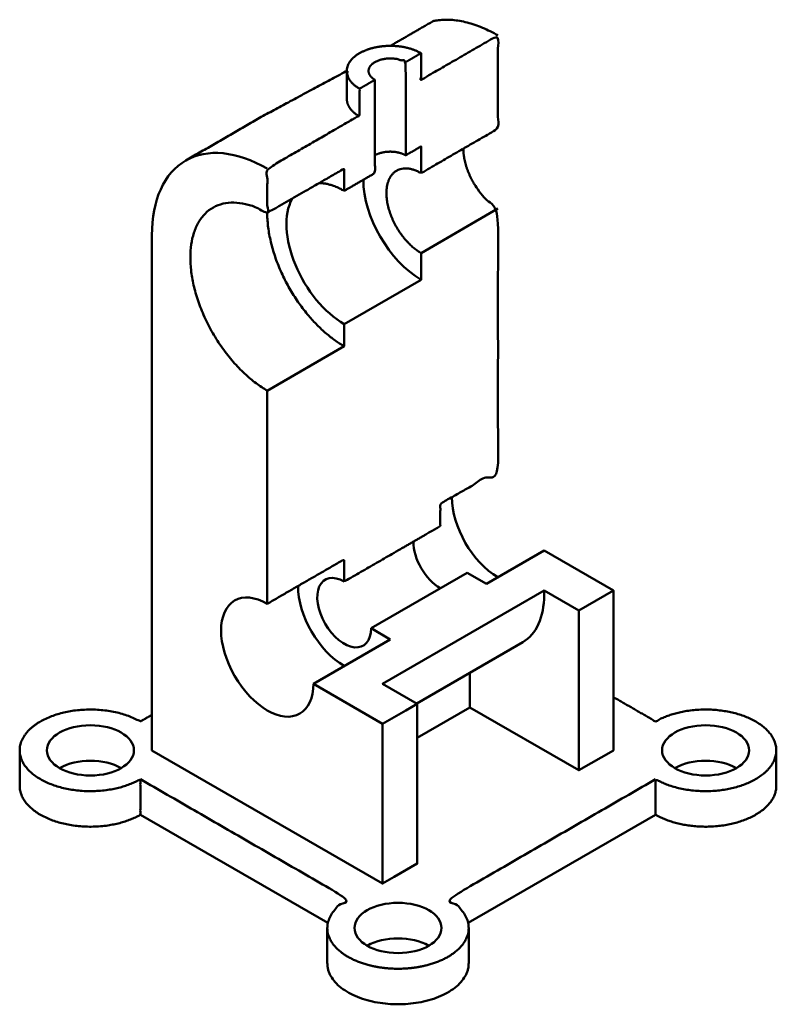
# Model space of a CAD drawing. Units: millimetres. Extents: x -222 to -52, y 145 to 366.
import ezdxf

# ---------------------------------------------------------------- set-up
doc = ezdxf.new("R2010")
doc.units = ezdxf.units.MM
doc.header["$MEASUREMENT"] = 0
doc.layers.add('M-OUTL', color=7, linetype='Continuous', lineweight=50)

msp = doc.modelspace()

# ---------------------------------------------------------------- linework, layer by layer
at = {"layer": 'M-OUTL'}
for p, q in [((-166.52, 282.95), (-166.52, 234.95)), ((-117.15, 239.45), (-104.16, 246.95)), ((-104.16, 246.95), (-88.57, 237.95)), ((-143.13, 229.45), (-121.48, 241.95)), ((-121.48, 241.95), (-117.15, 239.45)), ((-104.16, 237.95), (-96.37, 233.45)), ((-104.16, 236.95), (-104.16, 237.95)), ((-96.37, 233.45), (-96.37, 197.45)), ((-143.13, 229.45), (-138.8, 226.95)), ((-156.12, 216.95), (-138.8, 226.95)), ((-108.96, 226.31), (-132.85, 212.51)), ((-195.1, 187.45), (-152.87, 163.07)), ((-121.27, 163.07), (-79.05, 187.45))]:
    msp.add_line(p, q, dxfattribs=at)
for points in [[(-166.52, 272.95), (-166.52, 282.95), (-149.2, 292.95), (-149.2, 297.95), (-131.88, 307.95), (-131.88, 313.95), (-114.56, 323.95)], [(-140.54, 171.95), (-192.5, 201.95), (-192.5, 317.95)], [(-140.54, 207.95), (-135.34, 210.95), (-132.74, 212.45), (-140.54, 216.95), (-104.16, 237.95)], [(-96.37, 233.45), (-88.57, 237.95), (-88.57, 201.95), (-96.37, 197.45), (-120.91, 211.62)], [(-120.91, 219.41), (-120.91, 211.62), (-132.74, 204.78)], [(-135.34, 174.95), (-140.54, 171.95), (-140.54, 207.95), (-156.12, 216.95)], [(-132.74, 212.45), (-132.74, 176.45), (-137.94, 173.45)]]:
    msp.add_lwpolyline(points, dxfattribs=at)
for centre, major_axis, start_param, end_param in [((-166.52, 302.95), (18.37, -31.82), 2.356195, 3.141593), ((-166.52, 302.95), (18.37, -31.82), 3.141593, 3.92699), ((-131.88, 322.95), (9.19, -15.91), 3.926991, 5.497787), ((-149.2, 312.95), (9.19, -15.91), 3.48143, 5.497787), ((-114.56, 252.95), (7.35, -12.73), 3.926991, 5.497787), ((-127.55, 245.45), (4.29, -7.42), 3.926991, 5.497787), ((-149.2, 232.95), (4.29, -7.42), 2.356194, 7.068583), ((-149.2, 232.95), (7.35, -12.73), 3.926991, 5.497787), ((-166.52, 222.95), (7.35, -12.73), 3.141593, 6.283185), ((-166.52, 222.95), (7.35, -12.73), 2.356194, 3.141593), ((-120.62, 246.45), (-11.64, 20.15), 3.141593, 3.926986), ((-166.52, 222.95), (7.35, -12.73), 0, 0.785398), ((-206.35, 193.95), (-9.8, 0), 3.926991, 5.497787), ((-67.79, 193.95), (-9.8, 0), 3.926991, 5.497787), ((-137.07, 153.95), (-9.8, 0), 3.926991, 5.497787)]:
    msp.add_ellipse(centre, major_axis=major_axis, ratio=0.57735, start_param=start_param, end_param=end_param, dxfattribs=at)
for centre in [(-206.35, 201.95), (-67.79, 201.95), (-137.07, 161.95)]:
    msp.add_ellipse(centre, major_axis=(-9.8, 0), ratio=0.57735, dxfattribs=at)
for points, weights, knots in [([(-114.56, 362.95), (-122.52, 367.54), (-129.11, 366.2), (-133.96, 363.4), (-138.8, 360.6)], [1, 0.956124507826, 1, 1, 1], [0, 0, 0, 0.594644, 0.594644, 1.594644, 1.594644, 1.594644]), ([(-135.34, 356.95), (-133.61, 357.95), (-131.88, 358.95), (-131.88, 355.95), (-131.88, 352.95), (-123.22, 357.95), (-114.56, 362.95), (-114.56, 352.45), (-114.56, 341.95), (-123.22, 336.95), (-131.88, 331.95), (-136.38, 334.55), (-138.63, 331.34), (-140.88, 328.14), (-138.63, 322.34), (-136.38, 316.55), (-131.88, 313.95)], [1, 1, 1, 1, 1, 1, 1, 1, 1, 1, 1, 0.866025403784, 1, 0.866025403784, 1, 0.866025403784, 1], [0, 0, 0, 1, 1, 2, 2, 3, 3, 4, 4, 5, 5, 6.047198, 6.047198, 7.094395, 7.094395, 8.141593, 8.141593, 8.141593]), ([(-131.88, 358.95), (-135.88, 361.26), (-141.34, 360.41), (-146.8, 359.57), (-148.27, 356.41), (-149.73, 353.26), (-145.73, 350.95), (-145.73, 347.95), (-145.73, 344.95), (-156.12, 338.95), (-166.52, 332.95), (-166.52, 327.95), (-166.52, 322.95), (-183.84, 332.95), (-183.84, 312.95), (-183.84, 292.95), (-166.52, 282.95)], [1, 0.866025403784, 1, 0.866025403784, 1, 0.866025403784, 1, 1, 1, 1, 1, 1, 1, 0.707106781187, 1, 0.707106781187, 1], [0, 0, 0, 1.047198, 1.047198, 2.094395, 2.094395, 3.141593, 3.141593, 4.141593, 4.141593, 5.141593, 5.141593, 6.141593, 6.141593, 7.712389, 7.712389, 9.283185, 9.283185, 9.283185]), ([(-135.34, 335.95), (-135.34, 346.45), (-135.34, 356.95), (-137.34, 358.1), (-140.07, 357.68), (-142.8, 357.26), (-143.54, 355.68), (-144.27, 354.1), (-142.27, 352.95), (-144, 351.95), (-145.73, 350.95)], [1, 1, 1, 0.866025403784, 1, 0.866025403784, 1, 0.866025403784, 1, 1, 1], [0, 0, 0, 1, 1, 2.047198, 2.047198, 3.094395, 3.094395, 4.141593, 4.141593, 5.141593, 5.141593, 5.141593]), ([(-184.89, 334.77), (-176.23, 339.77), (-167.57, 344.77), (-167.24, 344.96), (-166.9, 345.13), (-157.75, 350.04), (-148.6, 354.95), (-148.6, 351.81), (-148.6, 348.68), (-148.6, 346.33), (-145.73, 344.68)], [1, 1, 1, 0.999840113738, 1, 1, 1, 1, 1, 0.923879532511, 1], [0, 0, 0, 1, 1, 1.035765, 1.035765, 2.035765, 2.035765, 3.035765, 3.035765, 3.821163, 3.821163, 3.821163]), ([(-142.27, 352.95), (-142.27, 349.95), (-142.27, 346.95), (-142.27, 339.45), (-142.27, 331.95), (-145.73, 329.95), (-149.2, 327.95), (-152.14, 329.65), (-154.79, 329.72)], [1, 1, 1, 1, 1, 1, 1, 0.975286862175, 1], [0, 0, 0, 1, 1, 2, 2, 3, 3, 3.445561, 3.445561, 3.445561]), ([(-122.35, 337.45), (-122.35, 333.72), (-120.07, 329.77), (-117.78, 325.81), (-114.56, 323.95), (-114.56, 294.45), (-114.56, 264.95), (-121.05, 261.2), (-127.55, 257.45), (-127.55, 254.95), (-127.55, 252.45), (-138.37, 246.2), (-149.2, 239.95), (-149.2, 242.45), (-149.2, 244.95), (-157.86, 239.95), (-166.52, 234.95)], [1, 0.923879532511, 1, 0.923879532511, 1, 1, 1, 1, 1, 1, 1, 1, 1, 1, 1, 1, 1], [0, 0, 0, 0.785398, 0.785398, 1.570796, 1.570796, 2.570796, 2.570796, 3.570796, 3.570796, 4.570796, 4.570796, 5.570796, 5.570796, 6.570796, 6.570796, 7.570796, 7.570796, 7.570796]), ([(-131.88, 331.95), (-131.88, 334.95), (-131.88, 337.95), (-133.61, 336.95), (-135.34, 335.95), (-136.77, 336.78), (-138.8, 336.78), (-140.83, 336.78), (-142.27, 335.95)], [1, 1, 1, 1, 1, 0.923879532511, 1, 0.923879532511, 1], [0, 0, 0, 1, 1, 2, 2, 2.785398, 2.785398, 3.570796, 3.570796, 3.570796]), ([(-149.2, 327.95), (-149.2, 330.45), (-149.2, 332.95), (-157.86, 327.95), (-166.52, 322.95), (-166.52, 314.66), (-161.44, 305.88), (-156.37, 297.09), (-149.2, 292.95)], [1, 1, 1, 1, 1, 0.923879532511, 1, 0.923879532511, 1], [0, 0, 0, 1, 1, 2, 2, 2.785398, 2.785398, 3.570796, 3.570796, 3.570796]), ([(-88.57, 213.95), (-83.81, 211.2), (-79.05, 208.45), (-71.53, 212.79), (-61.7, 210.44), (-51.87, 208.09), (-51.87, 201.95), (-51.87, 195.81), (-61.7, 193.46), (-71.53, 191.1), (-79.05, 195.45), (-79.05, 191.45), (-79.05, 187.45), (-71.52, 183.1), (-61.69, 185.46), (-51.86, 187.81), (-51.87, 193.95), (-51.87, 198.08), (-51.87, 202.2)], [1, 1, 1, 0.831469612303, 1, 0.831469612303, 1, 0.831469612303, 1, 0.831469612303, 1, 1, 1, 0.831409386962, 1, 0.831409386962, 1, 1, 1], [0, 0, 0, 1, 1, 2.178097, 2.178097, 3.356194, 3.356194, 4.534292, 4.534292, 5.712389, 5.712389, 6.712389, 6.712389, 7.890703, 7.890703, 9.069017, 9.069017, 10.069017, 10.069017, 10.069017]), ([(-222.25, 202.5), (-222.26, 198.24), (-222.28, 193.97), (-222.3, 187.82), (-212.46, 185.46), (-202.63, 183.1), (-195.1, 187.45), (-195.1, 191.45), (-195.1, 195.45), (-202.62, 191.1), (-212.45, 193.46), (-222.28, 195.81), (-222.28, 201.95), (-222.28, 208.09), (-212.45, 210.44), (-202.62, 212.79), (-195.1, 208.45), (-193.8, 209.2), (-192.5, 209.95)], [1, 1, 1, 0.831195038249, 1, 0.831195038249, 1, 1, 1, 0.831469612303, 1, 0.831469612303, 1, 0.831469612303, 1, 0.831469612303, 1, 1, 1], [0, 0, 0, 1, 1, 2.179085, 2.179085, 3.358171, 3.358171, 4.358171, 4.358171, 5.536268, 5.536268, 6.714365, 6.714365, 7.892462, 7.892462, 9.07056, 9.07056, 10.07056, 10.07056, 10.07056]), ([(-195.1, 195.45), (-171.71, 181.95), (-148.33, 168.45), (-155.85, 164.1), (-151.78, 158.43), (-147.71, 152.76), (-137.07, 152.76), (-126.43, 152.76), (-122.36, 158.43), (-118.29, 164.1), (-125.81, 168.45), (-102.43, 181.95), (-79.05, 195.45)], [1, 1, 1, 0.831469612303, 1, 0.831469612303, 1, 0.831469612303, 1, 0.831469612303, 1, 1, 1], [0, 0, 0, 1, 1, 2.178097, 2.178097, 3.356194, 3.356194, 4.534292, 4.534292, 5.712389, 5.712389, 6.712389, 6.712389, 6.712389]), ([(-152.99, 161.95), (-152.99, 157.95), (-152.99, 153.95), (-152.99, 144.76), (-137.07, 144.76), (-121.15, 144.76), (-121.15, 153.95), (-121.15, 157.95), (-121.15, 161.95)], [1, 1, 1, 0.707106781187, 1, 0.707106781187, 1, 1, 1], [0, 0, 0, 1, 1, 2.570796, 2.570796, 4.141593, 4.141593, 5.141593, 5.141593, 5.141593])]:
    msp.add_rational_spline(points, weights, degree=2, knots=knots, dxfattribs=at)

doc.saveas('drawing.dxf')
